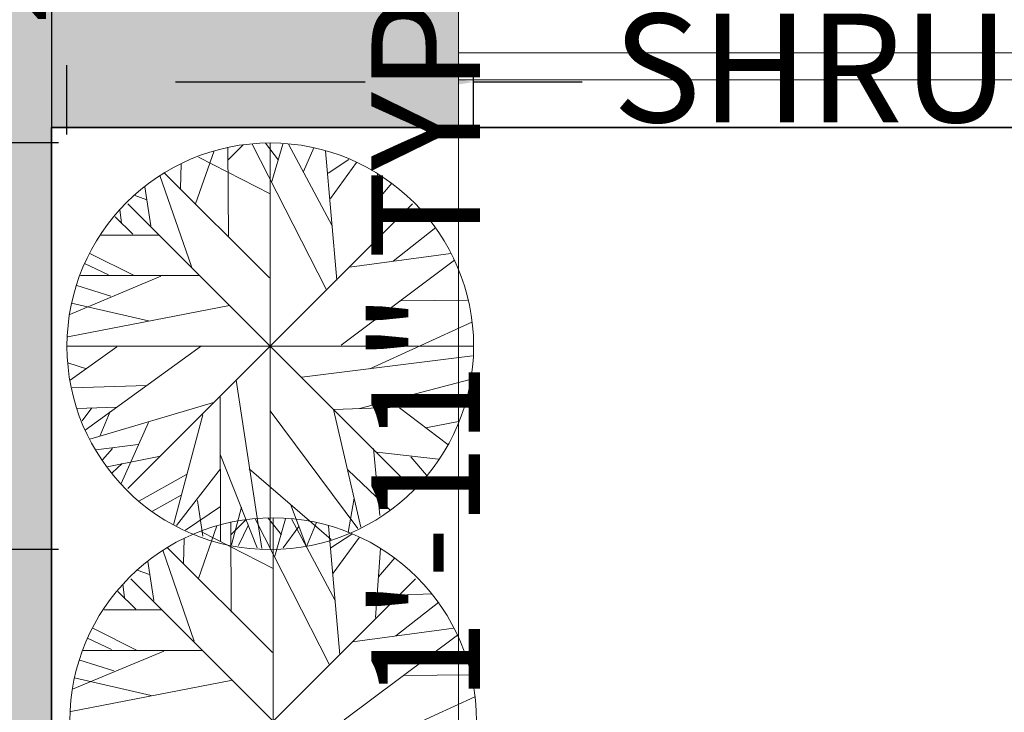
# Model space of a CAD drawing. Units: inches. Extents: x 2408 to 5087, y 2429 to 5085.
# Tile 3 of 12: x 2491 to 2564, y 2570 to 2622. Entities that reach past the tile are written whole.
import ezdxf

# ---------------------------------------------------------------- set-up
doc = ezdxf.new("R2010")
doc.units = ezdxf.units.IN
for name, color, linetype, lineweight in [('A-ANNO-DIMS', 2, 'Continuous', 18), ('A-GLAZ', 4, 'Continuous', 18), ('A-WALL', 7, 'Continuous', 35), ('A-WALL-PATT', 252, 'Continuous', 13), ('L-PLNT', 3, 'Continuous', 13)]:
    doc.layers.add(name, color=color, linetype=linetype, lineweight=lineweight)
doc.styles.get("Standard").update_dxf_attribs({"font": 'arial.ttf'})
doc.dimstyles.new('ISO-25', dxfattribs={"dimtxt": 8, "dimasz": 8, "dimexe": 1.25, "dimexo": 0.625, "dimtad": 0, "dimdec": 1, "dimlunit": 4, "dimtxsty": 'Standard', "dimcen": 2.5, "dimadec": 0, "dimazin": 0, "dimtfac": 1, "dimtdec": 1, "dimtmove": 0, "dimatfit": 3, "dimfxl": 1, "dimarcsym": 0})

# ---------------------------------------------------------------- blocks, each defined once
blk = doc.blocks.new('t2')
for p, q in [((3201.03, 2722), (3206.49, 2737.57)), ((3210.54, 2734.86), (3215.12, 2739.38)), ((3210.72, 2712.07), (3210.54, 2738.7)), ((3217.76, 2739.6), (3239.59, 2696.72)), ((3225.5, 2734.86), (3221.63, 2739.83)), ((3223.08, 2739.92), (3223.08, 2619.92)), ((3223.57, 2728.54), (3226.74, 2739.6)), ((3241.35, 2715.45), (3228.5, 2739.6)), ((3232.9, 2731.48), (3235.89, 2738.47)), ((3242.76, 2699.43), (3239.41, 2737.57)), ((3201.91, 2735.77), (3223.04, 2724.93)), ((3240.12, 2731.03), (3246.28, 2735.09)), ((3196.63, 2726.51), (3196.81, 2733.73)), ((3240.82, 2723.58), (3248.57, 2734.19)), ((3190.47, 2730.35), (3199.8, 2703.49)), ((3191.88, 2731.03), (3222.86, 2700.1)), ((3254.73, 2730.8), (3253.32, 2710.49)), ((3186.07, 2726.96), (3187.83, 2715.45)), ((3254.2, 2722.45), (3258.96, 2728.09)), ((3182.9, 2724.48), (3186.6, 2723.13)), ((3179.2, 2716.35), (3178.67, 2720.19)), ((3265.08, 2721.92), (3181.08, 2637.92)), ((3265.08, 2637.92), (3181.08, 2721.92)), ((3177.27, 2718.16), (3182.55, 2712.97)), ((3260.19, 2717.03), (3269.69, 2717.48)), ((3259.31, 2705.07), (3271.98, 2715)), ((3173.22, 2712.74), (3190.29, 2712.74)), ((3169.87, 2707.33), (3182.9, 2700.78)), ((3277.44, 2705.3), (3243.99, 2680.24)), ((3246.46, 2703.26), (3276.38, 2707.33)), ((3168.29, 2704.39), (3175.33, 2701.01)), ((3190.82, 2700.56), (3163.88, 2689.27)), ((3167.05, 2700.78), (3202.27, 2700.78)), ((3166, 2697.85), (3176.03, 2694.69)), ((3163.36, 2682.72), (3211.07, 2691.98)), ((3164.41, 2692.66), (3187.12, 2687.46)), ((3261.6, 2693.33), (3281.31, 2693.56)), ((3252.44, 2673.25), (3282.55, 2687.01)), ((3163.08, 2679.92), (3283.08, 2679.92)), ((3177.79, 2679.79), (3164.06, 2669.86)), ((3168.46, 2655.19), (3202.79, 2680.02)), ((3232.37, 2670.76), (3282.72, 2677.08)), ((3163.36, 2675.05), (3168.81, 2673.25)), ((3164.59, 2667.6), (3186.6, 2668.28)), ((3213, 2669.86), (3220.57, 2620.2)), ((3249.45, 2661.51), (3282.02, 2670.09)), ((3208.25, 2664.89), (3208.43, 2622.24)), ((3166, 2661.51), (3177.79, 2661.96)), ((3170.4, 2661.73), (3167.58, 2657.9)), ((3169.87, 2652.48), (3206.31, 2663.31)), ((3241.88, 2661.28), (3280.43, 2662.64)), ((3261.24, 2661.73), (3275.5, 2650.9)), ((3175.86, 2660.61), (3172.86, 2653.61)), ((3203.15, 2659.7), (3194.52, 2627.2)), ((3223.04, 2660.83), (3248.92, 2626.07)), ((3241.7, 2661.28), (3249.8, 2626.52)), ((3187.12, 2657.45), (3179.03, 2639.39)), ((3268.99, 2655.87), (3278.67, 2657.67)), ((3184.13, 2650.9), (3171.63, 2649.32)), ((3176.56, 2649.77), (3173.57, 2646.39)), ((3190.65, 2647.51), (3174.98, 2644.35)), ((3208.43, 2647.74), (3219.17, 2620.43)), ((3253.5, 2649.77), (3255.43, 2629.91)), ((3254.55, 2648.64), (3272.69, 2646.61)), ((3264.59, 2647.29), (3269.17, 2641.87)), ((3179.38, 2645.26), (3176.38, 2642.55)), ((3198.39, 2642.1), (3184.31, 2634.2)), ((3208.43, 2643.68), (3195.4, 2626.98)), ((3216.88, 2643.68), (3241, 2622.91)), ((3245.93, 2643.45), (3258.43, 2631.49)), ((3196.81, 2636), (3188.36, 2631.26)), ((3208.43, 2632.62), (3198.04, 2625.62)), ((3201.56, 2634.42), (3203.15, 2623.82)), ((3229.03, 2633.3), (3233.6, 2621.33)), ((3247.86, 2635.1), (3246.1, 2624.94)), ((3214.59, 2632.39), (3211.6, 2621.33)), ((3216.7, 2627.2), (3213.71, 2621.11)), ((3231.49, 2626.75), (3226.91, 2620.43))]:
    blk.add_line(p, q)
blk.add_circle((3223.08, 2679.92), 60)
blk = doc.blocks.new('WIN-60x9')
for p, q in [((3.5, 60), (3.5, 0)), ((5.5, 60), (5.5, 0))]:
    blk.add_line(p, q)
blk.add_lwpolyline([(0, 60), (9, 60), (9, 0), (0, 0)], close=True)
blk = doc.blocks.new('*D29')
at = {"layer": 'A-ANNO-DIMS', "color": 0, "lineweight": -2, "transparency": 16777216}
for p, q in [((2494.622, 2613.035), (2494.622, 2618.156)), ((2524.598, 2613.035), (2524.598, 2618.156)), ((2502.622, 2616.906), (2516.598, 2616.906)), ((2524.598, 2616.906), (2532.598, 2616.906))]:
    blk.add_line(p, q, dxfattribs=at)
at = {"layer": 'A-ANNO-DIMS', "color": 0, "transparency": 16777216}
for points in [[(2502.622, 2618.24), (2502.622, 2615.573), (2494.622, 2616.906)], [(2516.598, 2618.24), (2516.598, 2615.573), (2524.598, 2616.906)]]:
    blk.add_solid(points, dxfattribs=at)
at = {"layer": 'Defpoints', "color": 0, "transparency": 16777216}
for p in [(2524.598, 2616.906), (2494.622, 2612.41), (2524.598, 2612.41)]:
    blk.add_point(p, dxfattribs=at)
at = {"layer": 'A-ANNO-DIMS', "color": 0, "transparency": 16777216, "insert": (2578.699, 2616.906), "char_height": 8, "attachment_point": 5}
blk.add_mtext('SHRUB 2\'-6" TYP.', dxfattribs=at)
blk = doc.blocks.new('*D30')
at = {"layer": 'A-ANNO-DIMS', "color": 0, "lineweight": -2, "transparency": 16777216}
for p, q in [((2490.126, 2612.41), (2490.126, 2620.41)), ((2493.997, 2612.41), (2488.876, 2612.41)), ((2490.126, 2590.434), (2490.126, 2604.41)), ((2493.997, 2582.434), (2488.876, 2582.434))]:
    blk.add_line(p, q, dxfattribs=at)
at = {"layer": 'A-ANNO-DIMS', "color": 0, "transparency": 16777216}
for points in [[(2488.792, 2604.41), (2491.459, 2604.41), (2490.126, 2612.41)], [(2488.792, 2590.434), (2491.459, 2590.434), (2490.126, 2582.434)]]:
    blk.add_solid(points, dxfattribs=at)
at = {"layer": 'Defpoints', "color": 0, "transparency": 16777216}
for p in [(2490.126, 2612.41), (2494.622, 2612.41), (2494.622, 2582.434)]:
    blk.add_point(p, dxfattribs=at)
at = {"layer": 'A-ANNO-DIMS', "color": 0, "transparency": 16777216, "insert": (2490.126, 2645.485), "char_height": 8, "attachment_point": 5, "rotation": 90}
blk.add_mtext('2\'-6" TYP.', dxfattribs=at)
blk = doc.blocks.new('*D46')
at = {"layer": 'A-ANNO-DIMS', "color": 0, "lineweight": -2, "transparency": 16777216}
for p, q in [((2524.979, 2657.244), (2520.854, 2657.244)), ((2522.104, 2649.244), (2522.104, 2642.396)), ((2524.979, 2634.396), (2520.854, 2634.396)), ((2522.104, 2634.396), (2522.104, 2626.396))]:
    blk.add_line(p, q, dxfattribs=at)
at = {"layer": 'A-ANNO-DIMS', "color": 0, "transparency": 16777216}
for points in [[(2520.771, 2649.244), (2523.437, 2649.244), (2522.104, 2657.244)], [(2520.771, 2642.396), (2523.437, 2642.396), (2522.104, 2634.396)]]:
    blk.add_solid(points, dxfattribs=at)
at = {"layer": 'Defpoints', "color": 0, "transparency": 16777216}
for p in [(2525.604, 2657.244), (2522.104, 2634.396), (2525.604, 2634.396)]:
    blk.add_point(p, dxfattribs=at)
at = {"layer": 'A-ANNO-DIMS', "color": 0, "transparency": 16777216, "insert": (2522.104, 2598.657), "char_height": 8, "attachment_point": 5, "rotation": 90}
blk.add_mtext('1\'-11" TYP.', dxfattribs=at)
blk = doc.blocks.new('*D61')
at = {"layer": 'A-ANNO-DIMS', "color": 0, "lineweight": -2, "transparency": 16777216}
for p, q in [((2493.494, 2813.929), (2493.494, 2439.551)), ((2595.494, 2813.929), (2595.494, 2439.551)), ((2501.494, 2440.801), (2533.23, 2440.801)), ((2587.494, 2440.801), (2555.757, 2440.801))]:
    blk.add_line(p, q, dxfattribs=at)
at = {"layer": 'A-ANNO-DIMS', "color": 0, "transparency": 16777216}
for points in [[(2501.494, 2442.134), (2501.494, 2439.468), (2493.494, 2440.801)], [(2587.494, 2442.134), (2587.494, 2439.468), (2595.494, 2440.801)]]:
    blk.add_solid(points, dxfattribs=at)
at = {"layer": 'Defpoints', "color": 0, "transparency": 16777216}
for p in [(2493.494, 2814.554), (2595.494, 2814.554), (2595.494, 2440.801)]:
    blk.add_point(p, dxfattribs=at)
at = {"layer": 'A-ANNO-DIMS', "color": 0, "transparency": 16777216, "insert": (2544.494, 2440.801), "char_height": 8, "attachment_point": 5}
blk.add_mtext('8\'-6"', dxfattribs=at)

msp = doc.modelspace()

# ---------------------------------------------------------------- hatches: boundary and pattern name
at = {"layer": 'A-WALL-PATT'}
h = msp.add_hatch(color=256, dxfattribs=at)
h.dxf.hatch_style = 1
h.paths.add_polyline_path([(2493.494, 2613.554), (2523.494, 2613.554), (2523.494, 2622.554), (2493.494, 2622.554), (2493.494, 2714.804), (2484.494, 2714.804), (2484.494, 2497.751), (2493.494, 2497.751)])
h.paths.add_polyline_path([(2613.494, 2615.419), (2613.494, 2622.554), (2583.494, 2622.554), (2583.494, 2613.554), (2613.458, 2613.554, -0.009707)])
h.paths.add_polyline_path([(2823.494, 2634.554), (2814.494, 2634.554), (2814.494, 2622.554), (2694.494, 2622.554), (2694.494, 2670.554), (2706.494, 2670.554), (2706.494, 2675.054), (2694.494, 2675.054), (2694.494, 2750.054), (2685.494, 2750.054), (2685.494, 2622.554), (2661.494, 2622.554), (2661.494, 2613.554), (2814.494, 2613.554), (2814.494, 2522.054), (2688.494, 2522.054), (2688.494, 2513.054), (2823.494, 2513.054)])
h.paths.add_polyline_path([(2823.494, 2837.054), (2814.494, 2837.054), (2814.494, 2819.054), (2685.494, 2819.054), (2685.494, 2786.054), (2694.494, 2786.054), (2694.494, 2810.054), (2814.494, 2810.054), (2814.494, 2772.554), (2823.494, 2772.554)])
h.paths.add_polyline_path([(2694.494, 2964.554), (2595.494, 2964.554), (2595.494, 3008.054), (2601.494, 3008.054), (2601.494, 3017.054), (2484.494, 3017.054), (2484.494, 2972.054), (2493.494, 2972.054), (2493.494, 3008.054), (2586.494, 3008.054), (2586.494, 2955.554), (2685.494, 2955.554), (2685.494, 2854.87), (2694.494, 2854.87)])
h.paths.add_polyline_path([(2493.494, 2867.054), (2595.494, 2867.054), (2595.494, 2876.054), (2493.494, 2876.054), (2493.494, 2912.054), (2484.494, 2912.054), (2484.494, 2774.804), (2493.494, 2774.804)])
h.paths.add_polyline_path([(2595.494, 2814.554), (2493.494, 2814.554), (2493.494, 2810.054), (2595.494, 2810.054)], flags=17)
h.paths.add_polyline_path([(2724.494, 3017.054), (2625.494, 3017.054), (2625.494, 3008.054), (2685.494, 3008.054), (2685.494, 2994.554), (2694.494, 2994.554), (2694.494, 3008.054), (2724.494, 3008.054)])
h.paths.add_polyline_path([(2823.494, 3017.054), (2784.494, 3017.054), (2784.494, 3008.054), (2814.494, 3008.054), (2814.494, 2913.554), (2814.559, 2897.054), (2823.494, 2897.054)])
h.paths.add_polyline_path([(2823.494, 2712.554), (2814.613, 2712.554), (2814.658, 2701.271), (2814.494, 2701.271), (2814.494, 2675.054), (2740.994, 2675.054), (2740.994, 2687.054), (2736.494, 2687.054), (2736.494, 2670.554), (2814.494, 2670.554), (2814.494, 2658.554), (2823.494, 2658.554)], flags=17)

# ---------------------------------------------------------------- linework, layer by layer
at = {"layer": 'A-WALL'}
for p, q in [((2613.494, 2613.554), (2493.494, 2613.554)), ((2493.494, 2613.554), (2493.494, 2497.751))]:
    msp.add_line(p, q, dxfattribs=at)
at = {"layer": 'L-PLNT'}
msp.add_line((2523.494, 2613.554), (2523.494, 2506.751), dxfattribs=at)

# ---------------------------------------------------------------- block references
at = {"layer": 'A-GLAZ', "rotation": 269.9999999999976}
msp.add_blockref('WIN-60x9', (2523.494, 2622.554), dxfattribs=at)
at = {"layer": 'L-PLNT', "xscale": 0.2497966910751513, "yscale": 0.2497966910751513, "zscale": 0.2497966910751513}
for p in [(1704.496, 1927.986), (1704.709, 1900.351)]:
    msp.add_blockref('t2', p, dxfattribs=at)

# ---------------------------------------------------------------- dimensions: what is measured, and where the dimension line sits
at = {"layer": 'A-ANNO-DIMS'}
dim = msp.add_linear_dim(base=(2595.494, 2440.801), p1=(2493.494, 2814.554), p2=(2595.494, 2814.554), dimstyle='ISO-25', override={"dimdec": 1, "dimlfac": 1, "dimrnd": 0, "dimzin": 1, "dimdsep": 46, "dimlunit": 4, "dimfrac": 2}, dxfattribs=at)
dim.commit()
dim.dimension.update_dxf_attribs({"geometry": '*D61', "text_midpoint": (2544.494, 2440.801)})
for base, p1, p2, angle, picture, middle in [((2490.126, 2612.41), (2494.622, 2582.434), (2494.622, 2612.41), 90, '*D30', (2490.126, 2645.485)), ((2522.104, 2634.396), (2525.604, 2657.244), (2525.604, 2634.396), 270, '*D46', (2522.104, 2598.657))]:
    dim = msp.add_linear_dim(base=base, p1=p1, p2=p2, angle=angle, text='<> TYP.', dimstyle='ISO-25', override={"dimdec": 1, "dimlfac": 1, "dimrnd": 0, "dimzin": 1, "dimdsep": 46, "dimlunit": 4, "dimfrac": 2}, dxfattribs=at)
    dim.commit()
    dim.dimension.update_dxf_attribs({"geometry": picture, "text_midpoint": middle})
dim = msp.add_linear_dim(base=(2524.598, 2616.906), p1=(2494.622, 2612.41), p2=(2524.598, 2612.41), text='SHRUB <> TYP.', dimstyle='ISO-25', override={"dimdec": 1, "dimlfac": 1, "dimrnd": 0, "dimzin": 1, "dimdsep": 46, "dimlunit": 4, "dimfrac": 2}, dxfattribs=at)
dim.commit()
dim.dimension.update_dxf_attribs({"geometry": '*D29', "text_midpoint": (2578.699, 2616.906)})

doc.saveas('drawing.dxf')
